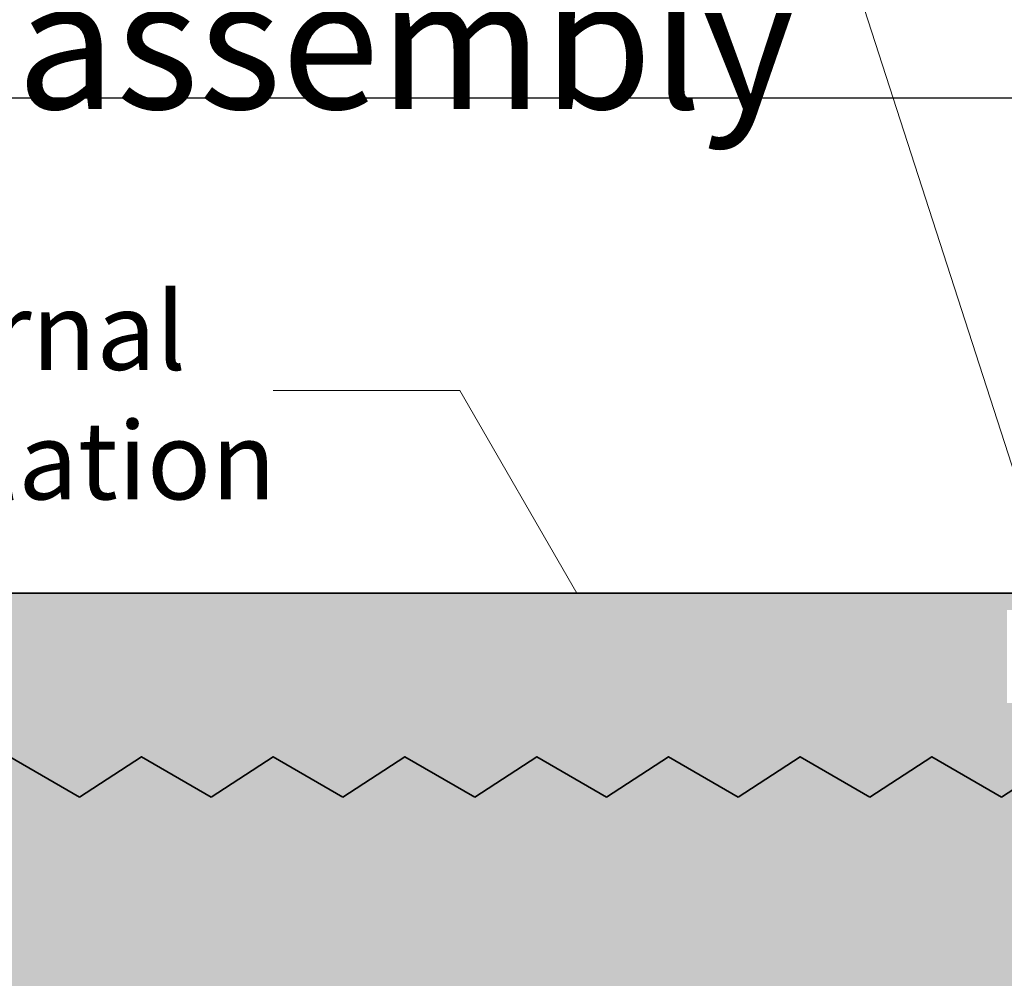
# Model space of a CAD drawing. Units: inches. Extents: x -1 to 292, y -3 to 199.
# Tile 22 of 52: x 68 to 106, y 93 to 130. Entities that reach past the tile are written whole.
import ezdxf

# ---------------------------------------------------------------- set-up
doc = ezdxf.new("R2010")
doc.units = ezdxf.units.IN
doc.header["$MEASUREMENT"] = 0
for name, color, linetype, lineweight in [('M-ANNO-LEAD', 2, 'Continuous', 18), ('M-ANNO-TEXT', 3, 'Continuous', 25), ('M-DIMS', 2, 'Continuous', 18), ('M-EQPM', 7, 'Continuous', 35), ('M-PATT', 8, 'Continuous', 13)]:
    doc.layers.add(name, color=color, linetype=linetype, lineweight=lineweight)
doc.styles.get("Standard").update_dxf_attribs({"font": 'arial.ttf'})
doc.dimstyles.get("Standard").update_dxf_attribs({"dimtxt": 0.18, "dimasz": 0.18, "dimexe": 0.18, "dimexo": 0.0625, "dimgap": 0.09, "dimtad": 0, "dimtih": 1, "dimtoh": 1, "dimdec": 4, "dimzin": 0, "dimdsep": 46, "dimtxsty": 'Standard', "dimcen": 0.09, "dimadec": 0, "dimazin": 0, "dimtfac": 1, "dimtdec": 4, "dimtofl": 0, "dimtmove": 0, "dimatfit": 3, "dimfxl": 1, "dimtolj": 1, "dimtzin": 0, "dimarcsym": 0})

# ---------------------------------------------------------------- blocks, each defined once
blk = doc.blocks.new('*D8')
at = {"layer": 'Defpoints', "color": 0, "transparency": 16777216}
for p in [(-0.662, 126.765), (111.488, 126.765), (69.013, 25.514)]:
    blk.add_point(p, dxfattribs=at)
at = {"layer": 'M-DIMS', "color": 0, "lineweight": -2, "transparency": 16777216}
for p, q in [((111.426, 126.765), (-0.842, 126.765)), ((-0.662, 126.585), (-0.662, 76.321)), ((-0.662, 25.694), (-0.662, 75.958)), ((68.951, 25.514), (-0.842, 25.514))]:
    blk.add_line(p, q, dxfattribs=at)
at = {"layer": 'M-DIMS', "color": 0, "transparency": 16777216}
for points in [[(-0.692, 126.585), (-0.632, 126.585), (-0.662, 126.765)], [(-0.692, 25.694), (-0.632, 25.694), (-0.662, 25.514)]]:
    blk.add_solid(points, dxfattribs=at)
at = {"layer": 'M-DIMS', "color": 0, "transparency": 16777216, "insert": (-0.662, 76.14), "char_height": 0.18, "attachment_point": 5}
blk.add_mtext('\\A1;101.25', dxfattribs=at)
blk = doc.blocks.new('*D9')
at = {"layer": 'Defpoints', "color": 0, "transparency": 16777216}
for p in [(177.053, 174.363), (49.924, 99.774), (177.053, 99.774)]:
    blk.add_point(p, dxfattribs=at)
at = {"layer": 'M-DIMS', "color": 0, "lineweight": -2, "transparency": 16777216}
for p, q in [((49.924, 99.836), (49.924, 174.543)), ((177.053, 99.836), (177.053, 174.543)), ((50.104, 174.363), (113.033, 174.363)), ((176.873, 174.363), (113.943, 174.363))]:
    blk.add_line(p, q, dxfattribs=at)
at = {"layer": 'M-DIMS', "color": 0, "transparency": 16777216}
for points in [[(50.104, 174.393), (50.104, 174.333), (49.924, 174.363)], [(176.873, 174.393), (176.873, 174.333), (177.053, 174.363)]]:
    blk.add_solid(points, dxfattribs=at)
at = {"layer": 'M-DIMS', "color": 0, "transparency": 16777216, "insert": (113.488, 174.363), "char_height": 0.18, "attachment_point": 5}
blk.add_mtext('\\A1;127.13', dxfattribs=at)

msp = doc.modelspace()

# ---------------------------------------------------------------- hatches: boundary and pattern name
at = {"layer": 'M-PATT'}
h = msp.add_hatch(color=256, dxfattribs=at)
h.set_gradient(color1=(237, 31, 36), color2=(242, 113, 114), tint=1, name='CYLINDER')
h.paths.add_polyline_path([(106.0735, 105.9941), (106.0735, 106.9941), (108.0603, 106.9941), (107.8488, 107.6501), (57.8007, 107.6501, 0.4142136), (49.9241, 99.7735), (52.3176, 101.3278), (55.0097, 99.7735), (57.4032, 101.3278), (60.0953, 99.7735), (62.4888, 101.3278), (65.1809, 99.7735), (67.5744, 101.3278), (70.2665, 99.7735), (72.66, 101.3278), (75.3521, 99.7735), (77.7456, 101.3278), (80.4377, 99.7735), (82.8312, 101.3278), (85.5233, 99.7735), (87.9168, 101.3278), (90.6089, 99.7735), (93.0024, 101.3278), (95.6945, 99.7735), (98.088, 101.3278), (100.7801, 99.7735), (103.1736, 101.3278), (105.8657, 99.7735), (108.2592, 101.3278), (110.9513, 99.7735), (113.3448, 101.3278), (116.0369, 99.7735), (118.4304, 101.3278), (121.1225, 99.7735), (123.516, 101.3278), (126.2082, 99.7735), (128.6016, 101.3278), (131.2938, 99.7735), (133.6872, 101.3278), (136.3794, 99.7735), (138.7728, 101.3278), (141.465, 99.7735), (143.8584, 101.3278), (146.5506, 99.7735), (148.944, 101.3278), (151.6362, 99.7735), (154.0296, 101.3278), (156.7218, 99.7735), (159.1152, 101.3278), (160.6222, 100.4578), (160.6222, 107.6501), (115.4883, 107.6501), (115.4883, 106.9941), (120.9032, 106.9941), (120.9032, 105.9941), (120.9032, 103.3981), (106.0735, 103.3981)])
h.paths.add_polyline_path([(169.176, 107.6501), (162.1623, 107.6501), (162.1623, 100.004), (164.2008, 101.3278), (166.893, 99.7735), (169.2864, 101.3278), (171.9786, 99.7735), (174.372, 101.3278), (177.0526, 99.7802, 0.4139642)])
h.paths.add_polyline_path([(111.4883, 107.6501), (107.8488, 107.6501), (108.0603, 106.9941), (111.4883, 106.9941)], flags=17)
h.paths.add_polyline_path([(61.6788, 91.897), (57.8007, 91.897, -0.1099266), (54.4604, 92.6403), (43.2011, 92.6403), (23.9502, 84.4688), (23.9502, 58.376), (43.2011, 47.2615), (50.9409, 47.2615, -0.2705926), (57.8007, 51.2672), (61.6788, 51.2672)])
h.paths.add_polyline_path([(73.6788, 91.897), (70.6788, 91.897), (70.6788, 51.2672), (73.6788, 51.2672)])
h.paths.add_polyline_path([(79.6788, 91.897), (76.6788, 91.897), (76.6788, 51.2672), (79.6788, 51.2672)])
h.paths.add_polyline_path([(67.6788, 91.897), (64.6788, 91.897), (64.6788, 51.2672), (67.6788, 51.2672)])
h.paths.add_polyline_path([(101.6788, 91.897), (82.6788, 91.897), (82.6788, 51.2672), (101.6788, 51.2672)])
h.paths.add_polyline_path([(107.6788, 91.897), (104.6788, 91.897), (104.6788, 51.2672), (107.6788, 51.2672)])
h.paths.add_polyline_path([(113.6788, 91.897), (110.6788, 91.897), (110.6788, 51.2672), (113.6788, 51.2672)])
h.paths.add_polyline_path([(119.6788, 91.897), (116.6788, 91.897), (116.6788, 51.2672), (119.6788, 51.2672)])
h.paths.add_polyline_path([(141.6788, 91.897), (122.6788, 91.897), (122.6788, 51.2672), (141.6788, 51.2672)])
h.paths.add_polyline_path([(147.6788, 91.897), (144.6788, 91.897), (144.6788, 51.2672), (147.6788, 51.2672)])
h.paths.add_polyline_path([(153.6788, 91.897), (150.6788, 91.897), (150.6788, 51.2672), (153.6788, 51.2672)])
h.paths.add_polyline_path([(159.6788, 91.897), (156.6788, 91.897), (156.6788, 51.2672), (159.6788, 51.2672)])
h.paths.add_polyline_path([(179.5897, 92.6403), (172.5163, 92.6403, -0.1099266), (169.176, 91.897), (162.6788, 91.897), (162.6788, 51.2672), (169.176, 51.2672, -0.2705926), (176.0358, 47.2615), (179.5897, 47.2615)])
h.paths.add_polyline_path([(203.0265, 84.4688), (183.7755, 92.6403), (181.5897, 92.6403), (181.5897, 47.2615), (183.7755, 47.2615), (203.0265, 58.376)])
h.paths.add_polyline_path([(184.4188, 61.52), (200.7224, 61.52), (200.7224, 77.7532), (184.4188, 77.7532)], flags=24)
h = msp.add_hatch(color=256, dxfattribs=at)
h.set_gradient(color1=(0, 255, 255), color2=(0, 255, 255), tint=1)
h.paths.add_polyline_path([(75.3521, 99.7735), (72.66, 101.3278), (70.2665, 99.7735), (67.5744, 101.3278), (65.1809, 99.7735), (62.4888, 101.3278), (60.0953, 99.7735), (57.4032, 101.3278), (55.0097, 99.7735), (52.3176, 101.3278), (49.9241, 99.7735, 0.4142136), (57.8007, 91.897), (61.6788, 91.897), (61.6788, 51.2672), (57.8007, 51.2672, 0.8088808), (54.5813, 36.2021), (65.0947, 51.2672), (64.6788, 51.2672), (64.6788, 91.897), (67.6788, 91.897), (67.6788, 51.2672), (65.0947, 51.2672), (54.5813, 36.2021, 0.1056561), (57.8007, 35.5141), (169.176, 35.5141, 1), (169.176, 51.2672), (162.6788, 51.2672), (162.6788, 91.897), (169.176, 91.897, 0.4144629), (177.0526, 99.7802), (174.372, 101.3278), (171.9786, 99.7735), (169.2864, 101.3278), (166.893, 99.7735), (164.2008, 101.3278), (162.1623, 100.004), (162.1623, 96.1027), (160.6222, 96.1027), (160.6222, 100.4578), (159.1152, 101.3278), (156.7218, 99.7735), (154.0296, 101.3278), (151.6362, 99.7735), (148.944, 101.3278), (146.5506, 99.7735), (143.8584, 101.3278), (141.465, 99.7735), (138.7728, 101.3278), (136.3794, 99.7735), (133.6872, 101.3278), (131.2938, 99.7735), (128.6016, 101.3278), (126.2082, 99.7735), (123.516, 101.3278), (121.1225, 99.7735), (118.4304, 101.3278), (116.0369, 99.7735), (113.3448, 101.3278), (110.9513, 99.7735), (108.2592, 101.3278), (105.8657, 99.7735), (103.1736, 101.3278), (100.7801, 99.7735), (98.088, 101.3278), (95.6945, 99.7735), (93.0024, 101.3278), (90.6089, 99.7735), (87.9168, 101.3278), (85.5233, 99.7735), (82.8312, 101.3278), (80.4377, 99.7735), (77.7456, 101.3278)])
h.paths.add_polyline_path([(79.6788, 91.897), (79.6788, 51.2672), (76.6788, 51.2672), (76.6788, 91.897)], flags=16)
h.paths.add_polyline_path([(73.6788, 91.897), (73.6788, 51.2672), (70.6788, 51.2672), (70.6788, 91.897)], flags=16)
h.paths.add_polyline_path([(82.6788, 91.897), (101.6788, 91.897), (101.6788, 51.2672), (82.6788, 51.2672)], flags=16)
h.paths.add_polyline_path([(104.6788, 91.897), (107.6788, 91.897), (107.6788, 51.2672), (104.6788, 51.2672)], flags=16)
h.paths.add_polyline_path([(110.6788, 91.897), (113.6788, 91.897), (113.6788, 51.2672), (110.6788, 51.2672)], flags=16)
h.paths.add_polyline_path([(116.6788, 91.897), (119.6788, 91.897), (119.6788, 51.2672), (116.6788, 51.2672)], flags=16)
h.paths.add_polyline_path([(122.6788, 91.897), (141.6788, 91.897), (141.6788, 51.2672), (144.6788, 51.2672), (144.6788, 91.897), (147.6788, 91.897), (147.6788, 51.2672), (122.6788, 51.2672)], flags=16)
h.paths.add_polyline_path([(150.6788, 91.897), (153.6788, 91.897), (153.6788, 51.2672), (150.6788, 51.2672)], flags=16)
h.paths.add_polyline_path([(156.6788, 91.897), (159.6788, 91.897), (159.6788, 51.2672), (156.6788, 51.2672)], flags=16)

# ---------------------------------------------------------------- linework, layer by layer
at = {"layer": 'M-ANNO-LEAD'}
for p, q in [((108.0603, 106.9941), (99.4422, 133.7141)), ((84.955, 115.473), (77.738, 115.473)), ((89.4716, 107.6501), (84.955, 115.473))]:
    msp.add_line(p, q, dxfattribs=at)
at = {"layer": 'M-EQPM'}
msp.add_lwpolyline([(110.9873, 107.6501), (57.8007, 107.6501, 1), (57.8007, 91.897), (61.6788, 91.897)], format="xyb", dxfattribs=at)
for points in [[(111.4883, 107.6501), (57.8007, 107.6501)], [(65.1809, 99.7735), (67.5744, 101.3278), (70.2665, 99.7735)], [(70.2665, 99.7735), (72.66, 101.3278), (75.3521, 99.7735)], [(75.3521, 99.7735), (77.7456, 101.3278), (80.4377, 99.7735)], [(80.4377, 99.7735), (82.8312, 101.3278), (85.5233, 99.7735)], [(85.5233, 99.7735), (87.9168, 101.3278), (90.6089, 99.7735)], [(90.6089, 99.7735), (93.0024, 101.3278), (95.6945, 99.7735)], [(95.6945, 99.7735), (98.088, 101.3278), (100.7801, 99.7735)], [(100.7801, 99.7735), (103.1736, 101.3278), (105.8657, 99.7735)], [(105.8657, 99.7735), (108.2592, 101.3278), (110.9513, 99.7735)]]:
    msp.add_lwpolyline(points, dxfattribs=at)

# ---------------------------------------------------------------- texts
at = {"layer": 'M-ANNO-TEXT', "attachment_point": 1}
for s, width, insert, char_height in [('mist pad \\Passembly', 40.442607, (67.8309, 139.6846), 5), ('external \\Pinsulation', 47.899539, (58.713, 119.2686), 3)]:
    msp.add_mtext_dynamic_manual_height_columns(s, width=width, gutter_width=1, heights=[0], dxfattribs=dict(at, insert=insert, char_height=char_height))

# ---------------------------------------------------------------- dimensions: what is measured, and where the dimension line sits
at = {"layer": 'M-DIMS'}
dim = msp.add_linear_dim(base=(177.0526, 174.3627), p1=(49.9241, 99.7735), p2=(177.0526, 99.7735), dimstyle='Standard', override={"dimdec": 2, "dimlfac": 1, "dimrnd": 0, "dimzin": 0, "dimdsep": 46, "dimlunit": 2}, dxfattribs=at)
dim.commit()
dim.dimension.update_dxf_attribs({"geometry": '*D9', "text_midpoint": (113.4883, 174.3627)})
dim = msp.add_linear_dim(base=(-0.6625, 126.765), p1=(69.013, 25.5141), p2=(111.4883, 126.765), angle=90, dimstyle='Standard', override={"dimdec": 2, "dimlfac": 1, "dimrnd": 0, "dimzin": 0, "dimdsep": 46, "dimlunit": 2}, dxfattribs=at)
dim.commit()
dim.dimension.update_dxf_attribs({"geometry": '*D8', "text_midpoint": (-0.6625, 76.1396)})

doc.saveas('drawing.dxf')
